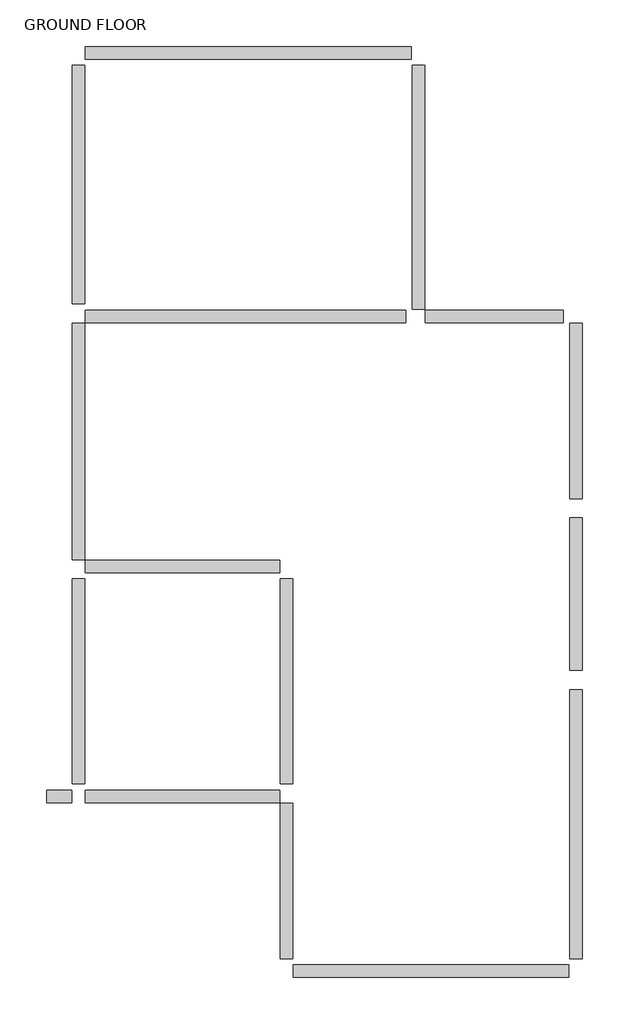
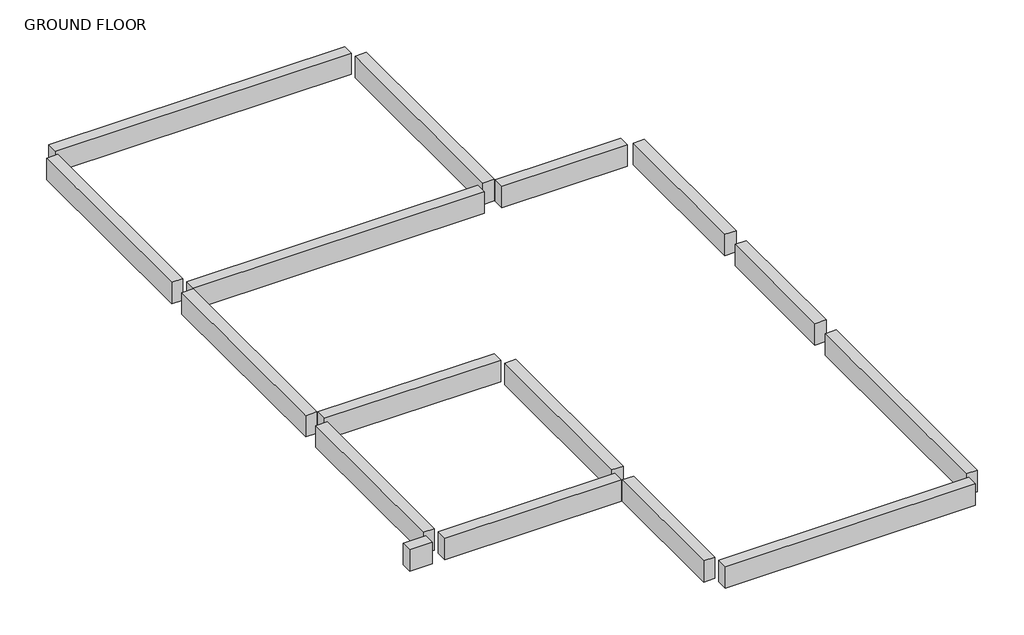
# One storey: 15 beams.
"""IFC4 building model written with IfcOpenShell, lengths in millimetres."""

from ifc_helpers import new_model, si_unit, frame, origin, place, context, project, spatial, polyline, outline, extrude, element, save

model = new_model("IFC4")

# Units and contexts
model_context = context("Model", 3, world=origin())
ifc_project = project(units=[si_unit("LENGTHUNIT", "METRE", prefix="MILLI")], contexts=[model_context])

# Site, building, storey
site = spatial("IfcSite", under=ifc_project)
building = spatial("IfcBuilding", under=site)
storey = spatial("IfcBuildingStorey", under=building, Name="GROUND FLOOR", Elevation=0.0)

# Beams
placement = place(None, origin())
element("IfcBeam", 1, ObjectType="Concrete-Rectangular Beam : 10\" x 24\"", at=placement, inside=storey, context=model_context, shape_type="SweptSolid", body=[
    extrude(outline(polyline([(-12235.0833659, 12888.2783402), (-12235.0833659, 13116.8783402), (-6266.0833659, 13116.8783402), (-6266.0833659, 12888.2783402), (-12235.0833659, 12888.2783402)])), frame((0.0, 0.0, -457.2), z_axis=(0.0, 0.0, 1.0), x_axis=(1.0, 0.0, 0.0)), (0.0, 0.0, 1.0), 457.2),
])
element("IfcBeam", 2, ObjectType="Concrete-Rectangular Beam : 10\" x 24\"", at=placement, inside=storey, context=model_context, shape_type="SweptSolid", body=[
    extrude(outline(polyline([(-6253.3833659, 12773.9783402), (-6024.7833659, 12773.9783402), (-6024.7833659, 8303.5783402), (-6253.3833659, 8303.5783402), (-6253.3833659, 12773.9783402)])), frame((0.0, 0.0, -457.2), z_axis=(0.0, 0.0, 1.0), x_axis=(1.0, 0.0, 0.0)), (0.0, 0.0, 1.0), 457.2),
])
element("IfcBeam", 3, ObjectType="Concrete-Rectangular Beam : 10\" x 24\"", at=placement, inside=storey, context=model_context, shape_type="SweptSolid", body=[
    extrude(outline(polyline([(-6012.0833659, 8062.2783402), (-6012.0833659, 8290.8783402), (-3484.7833659, 8290.8783402), (-3484.7833659, 8062.2783402), (-6012.0833659, 8062.2783402)])), frame((0.0, 0.0, -457.2), z_axis=(0.0, 0.0, 1.0), x_axis=(1.0, 0.0, 0.0)), (0.0, 0.0, 1.0), 457.2),
])
element("IfcBeam", 4, ObjectType="Concrete-Rectangular Beam : 10\" x 24\"", at=placement, inside=storey, context=model_context, shape_type="SweptSolid", body=[
    extrude(outline(polyline([(-3142.0191189, 4841.8494441), (-3370.6191189, 4841.8494441), (-3370.6191189, 8049.5783402), (-3142.0191189, 8049.5783402), (-3142.0191189, 4841.8494441)])), frame((0.0, 0.0, -457.2), z_axis=(0.0, 0.0, 1.0), x_axis=(1.0, 0.0, 0.0)), (0.0, 0.0, 1.0), 457.2),
])
element("IfcBeam", 5, ObjectType="Concrete-Rectangular Beam : 10\" x 24\"", at=placement, inside=storey, context=model_context, shape_type="SweptSolid", body=[
    extrude(outline(polyline([(-3142.0191189, 1700.3598175), (-3370.6191189, 1700.3598175), (-3370.6191189, 4486.2494441), (-3142.0191189, 4486.2494441), (-3142.0191189, 1700.3598175)])), frame((0.0, 0.0, -457.2), z_axis=(0.0, 0.0, 1.0), x_axis=(1.0, 0.0, 0.0)), (0.0, 0.0, 1.0), 457.2),
])
element("IfcBeam", 6, ObjectType="Concrete-Rectangular Beam : 10\" x 24\"", at=placement, inside=storey, context=model_context, shape_type="SweptSolid", body=[
    extrude(outline(polyline([(-3370.6191189, 1344.7598175), (-3142.0191189, 1344.7598175), (-3142.0191189, -3583.6216598), (-3370.6191189, -3583.6216598), (-3370.6191189, 1344.7598175)])), frame((0.0, 0.0, -457.2), z_axis=(0.0, 0.0, 1.0), x_axis=(1.0, 0.0, 0.0)), (0.0, 0.0, 1.0), 457.2),
])
element("IfcBeam", 7, ObjectType="Concrete-Rectangular Beam : 10\" x 24\"", at=placement, inside=storey, context=model_context, shape_type="SweptSolid", body=[
    extrude(outline(polyline([(-3383.3191189, -3697.9216598), (-3383.3191189, -3926.5216598), (-8425.0833659, -3926.5216598), (-8425.0833659, -3697.9216598), (-3383.3191189, -3697.9216598)])), frame((0.0, 0.0, -457.2), z_axis=(0.0, 0.0, 1.0), x_axis=(1.0, 0.0, 0.0)), (0.0, 0.0, 1.0), 457.2),
])
element("IfcBeam", 8, ObjectType="Concrete-Rectangular Beam : 10\" x 24\"", at=placement, inside=storey, context=model_context, shape_type="SweptSolid", body=[
    extrude(outline(polyline([(-8437.7833659, -3583.6216598), (-8666.3833659, -3583.6216598), (-8666.3833659, -738.8216598), (-8437.7833659, -738.8216598), (-8437.7833659, -3583.6216598)])), frame((0.0, 0.0, -457.2), z_axis=(0.0, 0.0, 1.0), x_axis=(1.0, 0.0, 0.0)), (0.0, 0.0, 1.0), 457.2),
])
element("IfcBeam", 9, ObjectType="Concrete-Rectangular Beam : 10\" x 24\"", at=placement, inside=storey, context=model_context, shape_type="SweptSolid", body=[
    extrude(outline(polyline([(-8666.3833659, 3369.6283402), (-8437.7833659, 3369.6283402), (-8437.7833659, -383.2216598), (-8666.3833659, -383.2216598), (-8666.3833659, 3369.6283402)])), frame((0.0, 0.0, -457.2), z_axis=(0.0, 0.0, 1.0), x_axis=(1.0, 0.0, 0.0)), (0.0, 0.0, 1.0), 457.2),
])
element("IfcBeam", 10, ObjectType="Concrete-Rectangular Beam : 10\" x 24\"", at=placement, inside=storey, context=model_context, shape_type="SweptSolid", body=[
    extrude(outline(polyline([(-12235.0833659, 3483.9283402), (-12235.0833659, 3712.5283402), (-8679.0833659, 3712.5283402), (-8679.0833659, 3483.9283402), (-12235.0833659, 3483.9283402)])), frame((0.0, 0.0, -457.2), z_axis=(0.0, 0.0, 1.0), x_axis=(1.0, 0.0, 0.0)), (0.0, 0.0, 1.0), 457.2),
])
element("IfcBeam", 11, ObjectType="Concrete-Rectangular Beam : 10\" x 24\"", at=placement, inside=storey, context=model_context, shape_type="SweptSolid", body=[
    extrude(outline(polyline([(-12247.7833659, -383.2216598), (-12476.3833659, -383.2216598), (-12476.3833659, 3369.6283402), (-12247.7833659, 3369.6283402), (-12247.7833659, -383.2216598)])), frame((0.0, 0.0, -457.2), z_axis=(0.0, 0.0, 1.0), x_axis=(1.0, 0.0, 0.0)), (0.0, 0.0, 1.0), 457.2),
])
element("IfcBeam", 12, ObjectType="Concrete-Rectangular Beam : 10\" x 24\"", at=placement, inside=storey, context=model_context, shape_type="SweptSolid", body=[
    extrude(outline(polyline([(-12946.2833659, -726.1216598), (-12946.2833659, -497.5216598), (-12489.0833659, -497.5216598), (-12489.0833659, -726.1216598), (-12946.2833659, -726.1216598)])), frame((0.0, 0.0, -457.2), z_axis=(0.0, 0.0, 1.0), x_axis=(1.0, 0.0, 0.0)), (0.0, 0.0, 1.0), 457.2),
    extrude(outline(polyline([(-8679.0833659, -497.5216598), (-8679.0833659, -726.1216598), (-12235.0833659, -726.1216598), (-12235.0833659, -497.5216598), (-8679.0833659, -497.5216598)])), frame((0.0, 0.0, -457.2), z_axis=(0.0, 0.0, 1.0), x_axis=(1.0, 0.0, 0.0)), (0.0, 0.0, 1.0), 457.2),
])
element("IfcBeam", 13, ObjectType="Concrete-Rectangular Beam : 10\" x 24\"", at=placement, inside=storey, context=model_context, shape_type="SweptSolid", body=[
    extrude(outline(polyline([(-12247.7833659, 3725.2283402), (-12476.3833659, 3725.2283402), (-12476.3833659, 8049.5783402), (-12247.7833659, 8049.5783402), (-12247.7833659, 3725.2283402)])), frame((0.0, 0.0, -457.2), z_axis=(0.0, 0.0, 1.0), x_axis=(1.0, 0.0, 0.0)), (0.0, 0.0, 1.0), 457.2),
])
element("IfcBeam", 14, ObjectType="Concrete-Rectangular Beam : 10\" x 24\"", at=placement, inside=storey, context=model_context, shape_type="SweptSolid", body=[
    extrude(outline(polyline([(-12247.7833659, 8405.1783402), (-12476.3833659, 8405.1783402), (-12476.3833659, 12773.9783402), (-12247.7833659, 12773.9783402), (-12247.7833659, 8405.1783402)])), frame((0.0, 0.0, -457.2), z_axis=(0.0, 0.0, 1.0), x_axis=(1.0, 0.0, 0.0)), (0.0, 0.0, 1.0), 457.2),
])
element("IfcBeam", 15, ObjectType="Concrete-Rectangular Beam : 10\" x 24\"", at=placement, inside=storey, context=model_context, shape_type="SweptSolid", body=[
    extrude(outline(polyline([(-6367.6833659, 8290.8783402), (-6367.6833659, 8062.2783402), (-12235.0833659, 8062.2783402), (-12235.0833659, 8290.8783402), (-6367.6833659, 8290.8783402)])), frame((0.0, 0.0, -457.2), z_axis=(0.0, 0.0, 1.0), x_axis=(1.0, 0.0, 0.0)), (0.0, 0.0, 1.0), 457.2),
])

save(model, "model.ifc")

# Revit data of these elements
# Type "Concrete-Rectangular Beam : 10\" x 24\""
#   Assembly Code = "B10"
#   Length [instance default] = 5' - 0"
#   b = 0' - 9"
#   h = 1' - 6"
#   Structural Material [instance default] = Concrete, Cast-in-Place gray
# Elements 1, 2, 3, 4, 5, 6, 7, 8, 9, 10, 11, 12, 13, 14, 15 (IfcBeam, "Concrete-Rectangular Beam : 10\" x 24\"")
#   Structural Material = Concrete, Cast-in-Place gray
#   Phase Created = New Construction
#   Materials on its faces: "Concrete, Cast-in-Place gray"
# Materials
#   "Concrete, Cast-in-Place gray": class "Concrete", colour RGB 192 192 192, transparency 0, Description = "Cast-in-place concrete", Cost = 0
